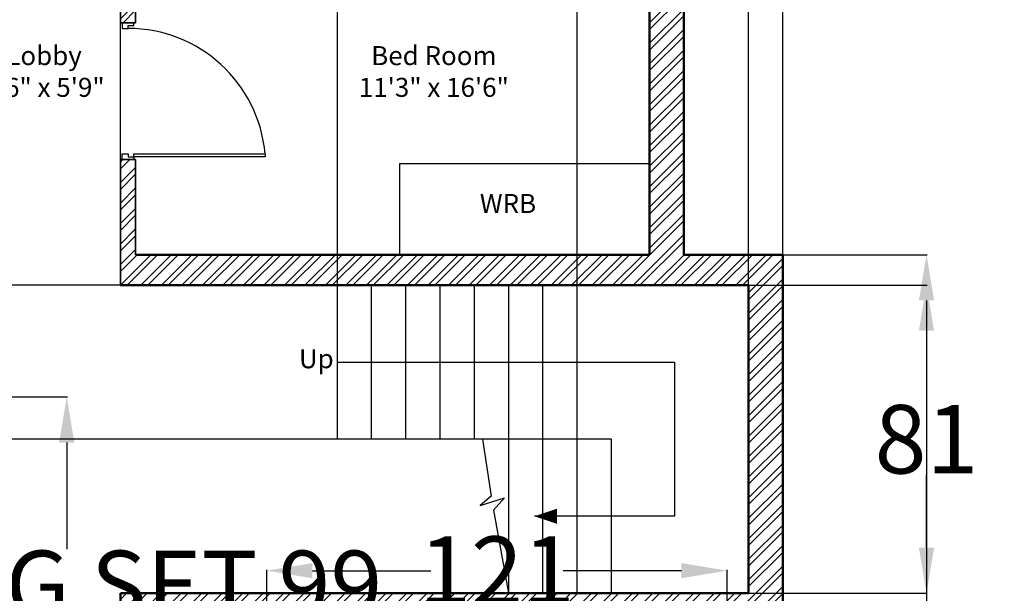
# Model space of a CAD drawing. Units: inches. Extents: x -90 to 536, y -553 to 299.
# Tile 22 of 27: x 207 to 465, y -153 to -2. Entities that reach past the tile are written whole.
import ezdxf

# ---------------------------------------------------------------- set-up
doc = ezdxf.new("R2010")
doc.units = ezdxf.units.IN
for name, color, linetype, lineweight in [('A-ANNO-DIMS', 2, 'Continuous', 18), ('A-ANNO-TEXT', 7, 'Continuous', 18), ('A-AREA-IDEN', 7, 'Continuous', 18), ('A-DOOR', 4, 'Continuous', 25), ('A-FLOR-CASE', 2, 'Continuous', 25), ('A-WALL-PATT', 252, 'Continuous', 13), ('Inner Wall', 5, 'Continuous', 35), ('Outer Wall', 1, 'Continuous', 50), ('Stairs', 8, 'Continuous', 25)]:
    doc.layers.add(name, color=color, linetype=linetype, lineweight=lineweight)
doc.styles.get("Standard").update_dxf_attribs({"font": 'arial.ttf'})
doc.dimstyles.get("Standard").update_dxf_attribs({"dimtxt": 18, "dimasz": 12, "dimexe": 0.18, "dimexo": 0.0625, "dimgap": 0.09, "dimtad": 0, "dimtih": 1, "dimtoh": 1, "dimdec": 0, "dimzin": 0, "dimdsep": 46, "dimlunit": 3, "dimtxsty": 'Standard', "dimcen": 0.09, "dimadec": 0, "dimazin": 0, "dimtfac": 1, "dimtdec": 0, "dimtofl": 0, "dimtmove": 0, "dimatfit": 3, "dimfxl": 1, "dimtolj": 1, "dimtzin": 0, "dimarcsym": 0})

# ---------------------------------------------------------------- blocks, each defined once
blk = doc.blocks.new('DOOR-36-A')
for points in [[(35.25, 37.5), (35.25, 3), (34.5, 3), (34.5, 37.5)], [(0, 0), (1.5, 0), (1.5, 1.5), (0.75, 1.5), (0.75, 3), (0, 3)], [(36, 0), (34.5, 0), (34.5, 1.5), (35.25, 1.5), (35.25, 3), (36, 3)]]:
    blk.add_lwpolyline(points, close=True)
blk.add_arc((37.64, 1.5), 36.14, 94.9791, 180)
blk = doc.blocks.new('WARDROBE')
blk.add_lwpolyline([(0, 65.56), (24, 65.56), (24, 0), (0, 0)], close=True)
blk = doc.blocks.new('*D41')
at = {"layer": 'A-ANNO-DIMS', "color": 0, "lineweight": -2, "transparency": 16777216}
for p, q in [((204.27, -100.92), (219.21, -100.92)), ((219.03, -112.92), (219.03, -140.95)), ((219.03, -187.77), (219.03, -159.74)), ((204.27, -199.77), (219.21, -199.77))]:
    blk.add_line(p, q, dxfattribs=at)
at = {"layer": 'A-ANNO-DIMS', "color": 0, "transparency": 16777216}
for points in [[(217.03, -112.92), (221.03, -112.92), (219.03, -100.92)], [(217.03, -187.77), (221.03, -187.77), (219.03, -199.77)]]:
    blk.add_solid(points, dxfattribs=at)
at = {"layer": 'Defpoints', "color": 0, "transparency": 16777216}
for p in [(204.21, -100.92), (219.03, -100.92), (204.21, -199.77)]:
    blk.add_point(p, dxfattribs=at)
at = {"layer": 'A-ANNO-DIMS', "color": 0, "transparency": 16777216, "insert": (219.03, -150.34), "char_height": 18, "attachment_point": 5}
blk.add_mtext('\\A1;DINING SET 99', dxfattribs=at)
blk = doc.blocks.new('*D44')
at = {"layer": 'A-ANNO-DIMS', "color": 0, "lineweight": -2, "transparency": 16777216}
for p, q in [((271.59, -173.44), (271.59, -146.42)), ((283.59, -146.6), (314.65, -146.6)), ((380.5, -146.6), (349.43, -146.6)), ((392.5, -173.44), (392.5, -146.42))]:
    blk.add_line(p, q, dxfattribs=at)
at = {"layer": 'A-ANNO-DIMS', "color": 0, "transparency": 16777216}
for points in [[(283.59, -144.6), (283.59, -148.6), (271.59, -146.6)], [(380.5, -144.6), (380.5, -148.6), (392.5, -146.6)]]:
    blk.add_solid(points, dxfattribs=at)
at = {"layer": 'Defpoints', "color": 0, "transparency": 16777216}
for p in [(392.5, -146.6), (271.59, -173.5), (392.5, -173.5)]:
    blk.add_point(p, dxfattribs=at)
at = {"layer": 'A-ANNO-DIMS', "color": 0, "transparency": 16777216, "insert": (332.04, -146.6), "char_height": 18, "attachment_point": 5}
blk.add_mtext('\\A1;121', dxfattribs=at)
blk = doc.blocks.new('*D53')
at = {"layer": 'A-ANNO-DIMS', "color": 0, "lineweight": -2, "transparency": 16777216}
for p, q in [((35.09, 103.75), (35.09, 287.38)), ((47.09, 287.2), (183.7, 287.2)), ((395.13, 287.2), (258.52, 287.2)), ((407.13, -63.49), (407.13, 287.38))]:
    blk.add_line(p, q, dxfattribs=at)
at = {"layer": 'A-ANNO-DIMS', "color": 0, "transparency": 16777216}
for points in [[(47.09, 289.2), (47.09, 285.2), (35.09, 287.2)], [(395.13, 289.2), (395.13, 285.2), (407.13, 287.2)]]:
    blk.add_solid(points, dxfattribs=at)
at = {"layer": 'Defpoints', "color": 0, "transparency": 16777216}
for p in [(407.13, 287.2), (35.09, 103.69), (407.13, -63.55)]:
    blk.add_point(p, dxfattribs=at)
at = {"layer": 'A-ANNO-DIMS', "color": 0, "transparency": 16777216, "insert": (221.11, 287.2), "char_height": 18, "attachment_point": 5}
blk.add_mtext('\\A1;372.04', dxfattribs=at)
blk = doc.blocks.new('*D55')
at = {"layer": 'A-ANNO-DIMS', "color": 0, "lineweight": -2, "transparency": 16777216}
for p, q in [((398.19, -71.55), (445.07, -71.55)), ((444.89, -83.55), (444.89, -102.77)), ((444.89, -140.55), (444.89, -121.33)), ((398.19, -152.55), (445.07, -152.55))]:
    blk.add_line(p, q, dxfattribs=at)
at = {"layer": 'A-ANNO-DIMS', "color": 0, "transparency": 16777216}
for points in [[(442.89, -83.55), (446.89, -83.55), (444.89, -71.55)], [(442.89, -140.55), (446.89, -140.55), (444.89, -152.55)]]:
    blk.add_solid(points, dxfattribs=at)
at = {"layer": 'Defpoints', "color": 0, "transparency": 16777216}
for p in [(398.13, -71.55), (398.13, -152.55), (444.89, -152.55)]:
    blk.add_point(p, dxfattribs=at)
at = {"layer": 'A-ANNO-DIMS', "color": 0, "transparency": 16777216, "insert": (444.89, -112.05), "char_height": 18, "attachment_point": 5}
blk.add_mtext('\\A1;81', dxfattribs=at)
blk = doc.blocks.new('*D58')
at = {"layer": 'A-ANNO-DIMS', "color": 0, "lineweight": -2, "transparency": 16777216}
for p, q in [((290.13, -71.49), (290.13, 287.38)), ((302.13, 287.2), (308.6, 287.2)), ((341.13, 287.2), (334.66, 287.2)), ((353.13, -71.49), (353.13, 287.38))]:
    blk.add_line(p, q, dxfattribs=at)
at = {"layer": 'A-ANNO-DIMS', "color": 0, "transparency": 16777216}
for points in [[(302.13, 289.2), (302.13, 285.2), (290.13, 287.2)], [(341.13, 289.2), (341.13, 285.2), (353.13, 287.2)]]:
    blk.add_solid(points, dxfattribs=at)
at = {"layer": 'Defpoints', "color": 0, "transparency": 16777216}
for p in [(353.13, 287.2), (290.13, -71.55), (353.13, -71.55)]:
    blk.add_point(p, dxfattribs=at)
at = {"layer": 'A-ANNO-DIMS', "color": 0, "transparency": 16777216, "insert": (321.63, 287.2), "char_height": 18, "attachment_point": 5}
blk.add_mtext('\\A1;63', dxfattribs=at)
blk = doc.blocks.new('*D59')
at = {"layer": 'A-ANNO-DIMS', "color": 0, "lineweight": -2, "transparency": 16777216}
for p, q in [((341.13174, 287.201217), (329.13174, 287.201217)), ((353.13174, -71.491283), (353.13174, 287.381217)), ((398.13174, -71.491283), (398.13174, 287.381217)), ((410.13174, 287.201217), (422.13174, 287.201217))]:
    blk.add_line(p, q, dxfattribs=at)
at = {"layer": 'A-ANNO-DIMS', "color": 0, "transparency": 16777216}
for points in [[(341.13174, 289.201217), (341.13174, 285.201217), (353.13174, 287.201217)], [(410.13174, 289.201217), (410.13174, 285.201217), (398.13174, 287.201217)]]:
    blk.add_solid(points, dxfattribs=at)
at = {"layer": 'Defpoints', "color": 0, "transparency": 16777216}
for p in [(398.13174, 287.201217), (353.13174, -71.553783), (398.13174, -71.553783)]:
    blk.add_point(p, dxfattribs=at)
at = {"layer": 'A-ANNO-DIMS', "color": 0, "transparency": 16777216, "insert": (375.63174, 287.201217), "char_height": 18, "attachment_point": 5}
blk.add_mtext('\\A1;45', dxfattribs=at)
blk = doc.blocks.new('*D60')
at = {"layer": 'A-ANNO-DIMS', "color": 0, "lineweight": -2, "transparency": 16777216}
for p, q in [((-2.67, -71.55), (-2.67, -59.55)), ((-2.67, -59.55), (9.33, -59.55)), ((290.07, -71.55), (-2.85, -71.55)), ((-2.67, -100.05), (-2.67, -83.55)), ((290.07, -112.05), (-2.85, -112.05))]:
    blk.add_line(p, q, dxfattribs=at)
at = {"layer": 'A-ANNO-DIMS', "color": 0, "transparency": 16777216}
for points in [[(-4.67, -83.55), (-0.67, -83.55), (-2.67, -71.55)], [(-4.67, -100.05), (-0.67, -100.05), (-2.67, -112.05)]]:
    blk.add_solid(points, dxfattribs=at)
at = {"layer": 'Defpoints', "color": 0, "transparency": 16777216}
for p in [(-2.67, -71.55), (290.13, -71.55), (290.13, -112.05)]:
    blk.add_point(p, dxfattribs=at)
at = {"layer": 'A-ANNO-DIMS', "color": 0, "transparency": 16777216, "insert": (33.23, -59.55), "char_height": 18, "attachment_point": 5}
blk.add_mtext('\\A1;40.5', dxfattribs=at)
blk = doc.blocks.new('*D62')
at = {"layer": 'A-ANNO-DIMS', "color": 0, "lineweight": -2, "transparency": 16777216}
for p, q in [((233.13, -71.49), (233.13, 287.38)), ((245.13, 287.2), (248.65, 287.2)), ((278.13, 287.2), (274.61, 287.2)), ((290.13, -71.49), (290.13, 287.38))]:
    blk.add_line(p, q, dxfattribs=at)
at = {"layer": 'A-ANNO-DIMS', "color": 0, "transparency": 16777216}
for points in [[(245.13, 289.2), (245.13, 285.2), (233.13, 287.2)], [(278.13, 289.2), (278.13, 285.2), (290.13, 287.2)]]:
    blk.add_solid(points, dxfattribs=at)
at = {"layer": 'Defpoints', "color": 0, "transparency": 16777216}
for p in [(290.13, 287.2), (233.13, -71.55), (290.13, -71.55)]:
    blk.add_point(p, dxfattribs=at)
at = {"layer": 'A-ANNO-DIMS', "color": 0, "transparency": 16777216, "insert": (261.63, 287.2), "char_height": 18, "attachment_point": 5}
blk.add_mtext('\\A1;57', dxfattribs=at)
blk = doc.blocks.new('*D68')
at = {"layer": 'A-ANNO-DIMS', "color": 0, "lineweight": -2, "transparency": 16777216}
for p, q in [((407.19, -63.55), (445.07, -63.55)), ((444.89, -75.55), (444.89, -211.27)), ((444.89, -365.55), (444.89, -229.84)), ((407.19, -377.55), (445.07, -377.55))]:
    blk.add_line(p, q, dxfattribs=at)
at = {"layer": 'A-ANNO-DIMS', "color": 0, "transparency": 16777216}
for points in [[(442.89, -75.55), (446.89, -75.55), (444.89, -63.55)], [(442.89, -365.55), (446.89, -365.55), (444.89, -377.55)]]:
    blk.add_solid(points, dxfattribs=at)
at = {"layer": 'Defpoints', "color": 0, "transparency": 16777216}
for p in [(407.13, -63.55), (407.13, -377.55), (444.89, -377.55)]:
    blk.add_point(p, dxfattribs=at)
at = {"layer": 'A-ANNO-DIMS', "color": 0, "transparency": 16777216, "insert": (444.89, -220.55), "char_height": 18, "attachment_point": 5}
blk.add_mtext('\\A1;314', dxfattribs=at)

msp = doc.modelspace()

# ---------------------------------------------------------------- hatches: boundary and pattern name
at = {"layer": 'A-WALL-PATT'}
h = msp.add_hatch(dxfattribs=at)
h.set_pattern_fill('ANSI32', color=256, scale=0.4)
h.set_pattern_definition([(45, (-88.8105, -603.6155), (-2.694077, 2.694077), []), (45, (-87.0145, -603.6155), (-2.694077, 2.694077), [])])
h.paths.add_polyline_path([(285.1317, 246.4462), (131.1317, 246.4462), (131.1317, 237.4462), (285.1317, 237.4462)])
h.paths.add_polyline_path([(122.1317, 237.4462), (113.1317, 237.4462), (113.1317, 152.4462), (122.1317, 152.4462), (122.1317, 166.4704)])
h.paths.add_polyline_path([(303.1317, 237.4462), (294.1317, 237.4462), (294.1317, 152.4462), (303.1317, 152.4462)])
h.paths.add_polyline_path([(47.1317, 91.9277), (38.1317, 91.9277), (38.1317, -6.5538), (77.1317, -6.5538), (77.1317, 2.4462), (70.5655, 2.4462), (47.1317, 2.4462)])
h.paths.add_polyline_path([(83.052, -61.5538), (47.1317, -61.5538), (47.1317, -24.5538), (38.1317, -24.5538), (38.1317, -70.5538), (74.052, -70.5538), (74.052, -223.5538), (38.1317, -223.5538), (38.1317, -503.5538), (92.1317, -503.5538), (92.1317, -437.5538), (191.1317, -437.5538), (191.1317, -428.5538), (83.1317, -428.5538), (83.1317, -494.5538), (47.1317, -494.5538), (47.1317, -232.5538), (83.052, -232.5538), (83.052, -70.5538)])
h.paths.add_polyline_path([(407.1317, -63.5538), (381.1317, -63.5538), (381.1317, 91.9277), (372.1317, 91.9277), (372.1317, 32.8805), (372.1317, -63.5538), (306.5745, -63.5538), (237.1317, -63.5538), (237.1317, -38.5538), (233.1317, -38.5538), (233.1317, -71.5538), (398.1317, -71.5538), (398.1317, -152.5538), (233.1317, -152.5538), (233.1317, -161.5538), (398.1317, -161.5538), (398.1317, -368.5538), (233.1317, -368.5538), (233.1317, -377.5538), (407.1317, -377.5538), (407.1317, -161.5538)])
h.paths.add_polyline_path([(261.1317, -422.5538), (252.1317, -422.5538), (252.1317, -428.5538), (233.1317, -428.5538), (233.1317, -437.5538), (261.1317, -437.5538)])
h.paths.add_polyline_path([(191.1317, -368.5538), (180.1317, -368.5538), (180.1317, -335.5538), (131.5919, -335.5538), (131.5919, -344.5538), (171.1317, -344.5538), (171.1317, -392.5538), (180.1317, -392.5538), (180.1317, -377.5538), (191.1317, -377.5538)], flags=17)
h.paths.add_polyline_path([(180.1317, -223.5538), (152.1317, -223.5538), (152.1317, -227.5538), (176.1317, -227.5538), (176.1317, -335.5538), (180.1317, -335.5538)], flags=17)
h.paths.add_polyline_path([(131.5919, -335.5538), (83.1317, -335.5538), (83.1317, -339.5538), (83.1317, -392.5538), (87.1317, -392.5538), (87.1317, -339.5538), (131.5919, -339.5538)], flags=17)
h.paths.add_polyline_path([(197.1317, 2.4462), (77.1317, 2.4462), (77.1317, -1.5538), (113.1317, -1.5538), (113.1317, -71.5538), (181.1317, -71.5538), (181.1317, -67.5538), (117.1317, -67.5538), (117.1317, -1.5538), (177.1317, -1.5538), (177.1317, -37.5538), (181.1317, -37.5538), (181.1317, -1.5538), (197.1317, -1.5538)])
h.paths.add_polyline_path([(173.1317, 138.4462), (122.1317, 138.4462), (122.1317, 134.4462), (173.1317, 134.4462)])
h.paths.add_polyline_path([(213.1317, 237.4462), (209.1317, 237.4462), (209.1317, 134.4462), (233.1317, 134.4462), (233.1317, 68.8889), (233.1317, -2.5538), (237.1317, -2.5538), (237.1317, 134.4462), (258.1317, 134.4462), (258.1317, 138.4462), (213.1317, 138.4462)])

# ---------------------------------------------------------------- linework, layer by layer
at = {"layer": 'Inner Wall'}
for p, q in [((233.1317, 134.4462), (233.1317, -2.5538)), ((237.1317, 134.4462), (237.1317, -2.5538)), ((233.1317, -2.5538), (237.1317, -2.5538)), ((233.1317, -38.5538), (237.1317, -38.5538)), ((233.1317, -38.5538), (233.1317, -71.5538)), ((237.1317, -38.5538), (237.1317, -63.5538))]:
    msp.add_line(p, q, dxfattribs=at)
at = {"layer": 'Outer Wall'}
for p, q in [((372.1317, 134.4462), (372.1317, -63.5538)), ((381.1317, 91.9277), (381.1317, -63.5538)), ((372.1317, -63.5538), (237.1317, -63.5538)), ((407.1317, -63.5538), (381.1317, -63.5538)), ((407.1317, -161.5538), (407.1317, -63.5538)), ((398.1317, -71.5538), (233.1317, -71.5538)), ((398.1317, -152.5538), (398.1317, -71.5538)), ((398.1317, -152.5538), (233.1317, -152.5538)), ((233.1317, -161.5538), (233.1317, -152.5538))]:
    msp.add_line(p, q, dxfattribs=at)
at = {"layer": 'Stairs'}
for p, q in [((290.1317, -112.0538), (290.1317, -71.5538)), ((299.1317, -112.0538), (299.1317, -71.5538)), ((308.1317, -112.0538), (308.1317, -71.5538)), ((317.1317, -112.0538), (317.1317, -71.5538)), ((326.1317, -112.0538), (326.1317, -71.5538)), ((335.1317, -112.0538), (335.1317, -71.5538)), ((344.1317, -112.0538), (344.1317, -71.5538)), ((353.1317, -112.0538), (353.1317, -71.5538)), ((290.1317, -91.8038), (378.698, -91.8038)), ((378.698, -91.8038), (378.698, -132.3038)), ((362.1317, -112.0538), (290.1317, -112.0538)), ((328.2499, -112.0538), (330.5452, -126.9888)), ((335.1317, -152.5538), (335.1317, -112.0538)), ((344.1317, -152.5538), (344.1317, -112.0538)), ((353.1317, -152.5538), (353.1317, -112.0538)), ((362.1317, -152.5538), (362.1317, -112.0538)), ((330.5452, -126.9888), (327.6325, -129.4977)), ((327.6325, -129.4977), (334.0109, -127.4472)), ((334.0109, -127.4472), (331.115, -130.6957)), ((331.115, -130.6957), (335.0949, -152.5538)), ((378.698, -132.3038), (341.8802, -132.3038))]:
    msp.add_line(p, q, dxfattribs=at)
msp.add_lwpolyline([(341.8802, -132.3038, 0, 4, 0), (347.8428, -132.3038, 4, 4, 0)], format="xyseb", dxfattribs=at)

# ---------------------------------------------------------------- block references
at = {"layer": 'A-DOOR', "rotation": 269.9999999999998}
msp.add_blockref('DOOR-36-A', (233.6317, -2.5538), dxfattribs=at)
at = {"layer": 'A-FLOR-CASE', "rotation": 270.0000000000001}
msp.add_blockref('WARDROBE', (306.5745, -39.5538), dxfattribs=at)

# ---------------------------------------------------------------- texts
at = {"layer": 'A-ANNO-TEXT', "char_height": 5, "attachment_point": 3}
for s, width, insert in [('\\pxqc;{\\fTimes New Roman|b0|i0|c0|p18;WRB}', 35.23368, (352.5618, -47.5786)), ('\\pxqc;{\\fTimes New Roman|b0|i0|c0|p18;Up}', 49.342153, (309.2667, -88.3815))]:
    msp.add_mtext_dynamic_manual_height_columns(s, width=width, gutter_width=12.5, heights=[0], dxfattribs=dict(at, insert=insert))
at = {"layer": 'A-AREA-IDEN', "char_height": 5, "attachment_point": 3}
for s, insert in [('\\pxqc;{\\fTimes New Roman|b0|i0|c0|p18;Lobby\\P4\'6" x 5\'9"}', (237.7373, -8.7077)), ('\\pxqc;{\\fTimes New Roman|b0|i0|c0|p18;Bed Room\\P11\'3" x 16\'6"}', (340.1454, -8.7077))]:
    msp.add_mtext_dynamic_manual_height_columns(s, width=49.342153, gutter_width=12.5, heights=[0], dxfattribs=dict(at, insert=insert))

# ---------------------------------------------------------------- dimensions: what is measured, and where the dimension line sits
at = {"layer": 'A-ANNO-DIMS'}
for base, p1, p2, override, picture, middle in [((407.1317, 287.2012), (35.0873, 103.6916), (407.1317, -63.5538), {"dimdec": 2, "dimlfac": 1, "dimrnd": 0, "dimzin": 0, "dimdsep": 46, "dimlunit": 2}, '*D53', (221.1095, 287.2012)), ((290.1317, 287.2012), (233.1317, -71.5538), (290.1317, -71.5538), {"dimdec": 0, "dimlfac": 1, "dimrnd": 0, "dimzin": 0, "dimdsep": 46, "dimlunit": 2}, '*D62', (261.6317, 287.2012)), ((353.1317, 287.2012), (290.1317, -71.5538), (353.1317, -71.5538), {"dimdec": 0, "dimlfac": 1, "dimrnd": 0, "dimzin": 0, "dimdsep": 46, "dimlunit": 2}, '*D58', (321.6317, 287.2012)), ((398.1317, 287.2012), (353.1317, -71.5538), (398.1317, -71.5538), {"dimdec": 0, "dimlfac": 1, "dimrnd": 0, "dimzin": 0, "dimdsep": 46, "dimlunit": 2}, '*D59', (375.6317, 287.2012)), ((392.4952, -146.6021), (271.5922, -173.4988), (392.4952, -173.4988), {"dimdec": 0, "dimlfac": 1, "dimrnd": 0, "dimzin": 0, "dimdsep": 46, "dimlunit": 2}, '*D44', (332.0437, -146.6021))]:
    dim = msp.add_linear_dim(base=base, p1=p1, p2=p2, dimstyle='Standard', override=override, dxfattribs=at)
    dim.commit()
    dim.dimension.update_dxf_attribs({"geometry": picture, "text_midpoint": middle})
for base, p1, p2, override, picture, middle in [((-2.6677, -71.5538), (290.1317, -112.0538), (290.1317, -71.5538), {"dimdec": 1, "dimlfac": 1, "dimrnd": 0, "dimzin": 0, "dimdsep": 46, "dimlunit": 2}, '*D60', (33.2299, -59.5538)), ((444.8867, -377.5538), (407.1317, -63.5538), (407.1317, -377.5538), {"dimdec": 0, "dimlfac": 1, "dimrnd": 0, "dimzin": 0, "dimdsep": 46, "dimlunit": 2}, '*D68', (444.8867, -220.5538)), ((444.8867, -152.5538), (398.1317, -71.5538), (398.1317, -152.5538), {"dimdec": 0, "dimlfac": 1, "dimrnd": 0, "dimzin": 0, "dimdsep": 46, "dimlunit": 2}, '*D55', (444.8867, -112.0538))]:
    dim = msp.add_linear_dim(base=base, p1=p1, p2=p2, angle=90, dimstyle='Standard', override=override, dxfattribs=at)
    dim.commit()
    dim.dimension.update_dxf_attribs({"geometry": picture, "text_midpoint": middle})
dim = msp.add_linear_dim(base=(219.0345, -100.9205), p1=(204.2077, -199.766), p2=(204.2077, -100.9205), angle=90, text='DINING SET <>', dimstyle='Standard', override={"dimdec": 0, "dimlfac": 1, "dimrnd": 0, "dimzin": 0, "dimdsep": 46, "dimlunit": 2}, dxfattribs=at)
dim.commit()
dim.dimension.update_dxf_attribs({"geometry": '*D41', "text_midpoint": (219.0345, -150.3432)})

doc.saveas('drawing.dxf')
